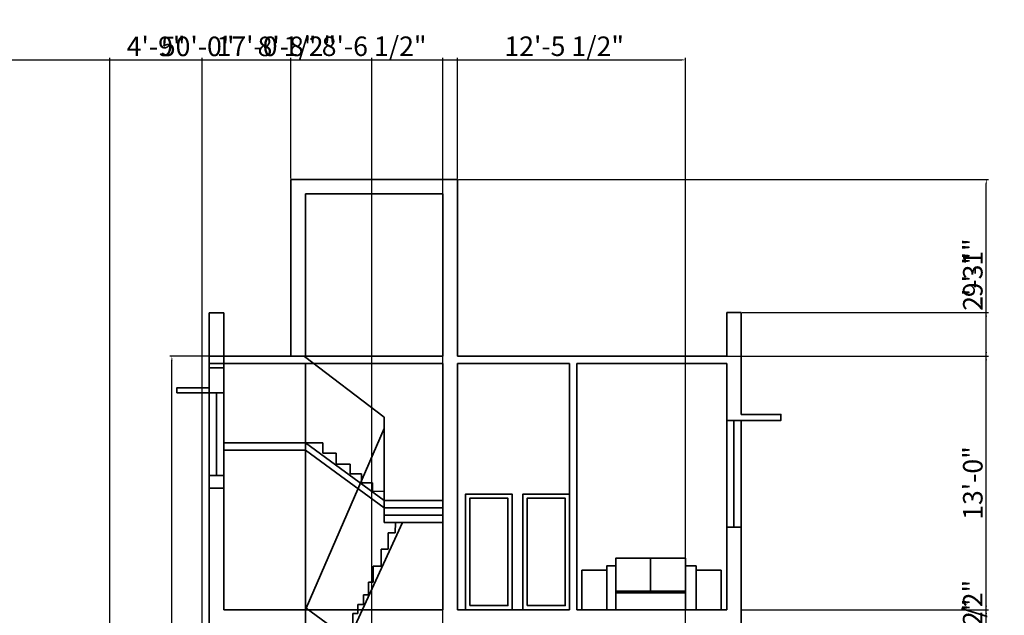
# Model space of a CAD drawing. Units: inches. Extents: x 1367 to 2309, y 1406 to 3826.
# Tile 9 of 9: x 1704 to 2309, y 3460 to 3826. Entities that reach past the tile are written whole.
import ezdxf

# ---------------------------------------------------------------- set-up
doc = ezdxf.new("R2010")
doc.units = ezdxf.units.IN
doc.layers.add('A-ANNO-DIMS', color=2, linetype='Continuous', lineweight=18)
doc.layers.add('A-SECT', color=7, linetype='Continuous', lineweight=35)
doc.styles.get("Standard").update_dxf_attribs({"font": 'arial.ttf'})
doc.dimstyles.new('ISO-25', dxfattribs={"dimtxt": 12, "dimasz": 2.5, "dimexe": 1.25, "dimexo": 0.625, "dimtad": 1, "dimdec": 0, "dimlunit": 4, "dimtxsty": 'Standard', "dimcen": 2.5, "dimadec": 0, "dimazin": 0, "dimtfac": 1, "dimtdec": 0, "dimtmove": 0, "dimatfit": 3, "dimfxl": 1, "dimarcsym": 0})

# ---------------------------------------------------------------- blocks, each defined once
blk = doc.blocks.new('*D42')
at = {"layer": 'A-ANNO-DIMS', "color": 0, "lineweight": -2, "transparency": 16777216}
for p, q in [((1819.79, 3619.06), (1796.28, 3619.06)), ((1797.53, 3153.56), (1797.53, 3616.56)), ((1819.79, 3151.06), (1796.28, 3151.06))]:
    blk.add_line(p, q, dxfattribs=at)
at = {"layer": 'A-ANNO-DIMS', "color": 0, "lineweight": 100, "transparency": 16777216}
for points in [[(1797.12, 3616.56), (1797.95, 3616.56), (1797.53, 3619.06)], [(1797.12, 3153.56), (1797.95, 3153.56), (1797.53, 3151.06)]]:
    blk.add_solid(points, dxfattribs=at)
at = {"layer": 'Defpoints', "color": 0, "lineweight": 100, "transparency": 16777216}
for p in [(1797.53, 3619.06), (1820.42, 3619.06), (1820.42, 3151.06)]:
    blk.add_point(p, dxfattribs=at)
at = {"layer": 'A-ANNO-DIMS', "color": 0, "transparency": 16777216, "insert": (1790.78, 3385.06), "char_height": 12, "attachment_point": 5, "rotation": 90}
blk.add_mtext("39'", dxfattribs=at)
blk = doc.blocks.new('*D87')
at = {"layer": 'A-ANNO-DIMS', "color": 0, "lineweight": -2, "transparency": 16777216}
for p, q in [((1513.37, 2814.79), (1513.37, 3802.6)), ((2113.4, 2814.79), (2113.4, 3802.6)), ((1515.87, 3801.35), (2110.9, 3801.35))]:
    blk.add_line(p, q, dxfattribs=at)
at = {"layer": 'A-ANNO-DIMS', "color": 0, "lineweight": 100, "transparency": 16777216}
for points in [[(1515.87, 3801.77), (1515.87, 3800.93), (1513.37, 3801.35)], [(2110.9, 3801.77), (2110.9, 3800.93), (2113.4, 3801.35)]]:
    blk.add_solid(points, dxfattribs=at)
at = {"layer": 'Defpoints', "color": 0, "lineweight": 100, "transparency": 16777216}
for p in [(2113.4, 3801.35), (1513.37, 2814.17), (2113.4, 2814.17)]:
    blk.add_point(p, dxfattribs=at)
at = {"layer": 'A-ANNO-DIMS', "color": 0, "transparency": 16777216, "insert": (1813.39, 3808.1), "char_height": 12, "attachment_point": 5}
blk.add_mtext('50\'-0"', dxfattribs=at)
blk = doc.blocks.new('*D103')
at = {"layer": 'A-ANNO-DIMS', "color": 0, "lineweight": -2, "transparency": 16777216}
for p, q in [((1504.37, 3284.24), (1504.37, 3802.6)), ((1759.42, 3284.24), (1759.42, 3802.6)), ((1506.87, 3801.35), (1756.92, 3801.35))]:
    blk.add_line(p, q, dxfattribs=at)
at = {"layer": 'A-ANNO-DIMS', "color": 0, "lineweight": 100, "transparency": 16777216}
for points in [[(1506.87, 3801.77), (1506.87, 3800.93), (1504.37, 3801.35)], [(1756.92, 3801.77), (1756.92, 3800.93), (1759.42, 3801.35)]]:
    blk.add_solid(points, dxfattribs=at)
at = {"layer": 'Defpoints', "color": 0, "lineweight": 100, "transparency": 16777216}
for p in [(1759.42, 3801.35), (1504.37, 3283.62), (1759.42, 3283.62)]:
    blk.add_point(p, dxfattribs=at)
at = {"layer": 'A-ANNO-DIMS', "color": 0, "transparency": 16777216, "insert": (1631.89, 3808.1), "char_height": 12, "attachment_point": 5}
blk.add_mtext('21\'-3"', dxfattribs=at)
blk = doc.blocks.new('*D106')
at = {"layer": 'A-ANNO-DIMS', "color": 0, "lineweight": -2, "transparency": 16777216}
for p, q in [((1759.42, 3063.31), (1759.42, 3802.6)), ((1964.13, 3080.24), (1964.13, 3802.6)), ((1761.92, 3801.35), (1961.63, 3801.35))]:
    blk.add_line(p, q, dxfattribs=at)
at = {"layer": 'A-ANNO-DIMS', "color": 0, "lineweight": 100, "transparency": 16777216}
for points in [[(1761.92, 3801.77), (1761.92, 3800.93), (1759.42, 3801.35)], [(1961.63, 3801.77), (1961.63, 3800.93), (1964.13, 3801.35)]]:
    blk.add_solid(points, dxfattribs=at)
at = {"layer": 'Defpoints', "color": 0, "lineweight": 100, "transparency": 16777216}
for p in [(1964.13, 3801.35), (1964.13, 3079.62), (1759.42, 3062.68)]:
    blk.add_point(p, dxfattribs=at)
at = {"layer": 'A-ANNO-DIMS', "color": 0, "transparency": 16777216, "insert": (1861.77, 3808.18), "char_height": 12, "attachment_point": 5}
blk.add_mtext('17\'-0 1/2"', dxfattribs=at)
blk = doc.blocks.new('*D107')
at = {"layer": 'A-ANNO-DIMS', "color": 0, "lineweight": -2, "transparency": 16777216}
for p, q in [((1964.13, 3080.24), (1964.13, 3802.6)), ((2113.4, 3080.24), (2113.4, 3802.6)), ((1966.63, 3801.35), (2110.9, 3801.35))]:
    blk.add_line(p, q, dxfattribs=at)
at = {"layer": 'A-ANNO-DIMS', "color": 0, "lineweight": 100, "transparency": 16777216}
for points in [[(1966.63, 3801.77), (1966.63, 3800.93), (1964.13, 3801.35)], [(2110.9, 3801.77), (2110.9, 3800.93), (2113.4, 3801.35)]]:
    blk.add_solid(points, dxfattribs=at)
at = {"layer": 'Defpoints', "color": 0, "lineweight": 100, "transparency": 16777216}
for p in [(2113.4, 3801.35), (1964.13, 3079.62), (2113.4, 3079.62)]:
    blk.add_point(p, dxfattribs=at)
at = {"layer": 'A-ANNO-DIMS', "color": 0, "transparency": 16777216, "insert": (2038.76, 3808.18), "char_height": 12, "attachment_point": 5}
blk.add_mtext('12\'-5 1/2"', dxfattribs=at)
blk = doc.blocks.new('*D110')
at = {"layer": 'A-ANNO-DIMS', "color": 0, "lineweight": -2, "transparency": 16777216}
for p, q in [((1816.25, 3045.71), (1816.25, 3802.6)), ((1920.42, 3047.12), (1920.42, 3802.6)), ((1818.75, 3801.35), (1917.92, 3801.35))]:
    blk.add_line(p, q, dxfattribs=at)
at = {"layer": 'A-ANNO-DIMS', "color": 0, "lineweight": 100, "transparency": 16777216}
for points in [[(1818.75, 3801.77), (1818.75, 3800.93), (1816.25, 3801.35)], [(1917.92, 3801.77), (1917.92, 3800.93), (1920.42, 3801.35)]]:
    blk.add_solid(points, dxfattribs=at)
at = {"layer": 'Defpoints', "color": 0, "lineweight": 100, "transparency": 16777216}
for p in [(1920.42, 3801.35), (1816.25, 3045.09), (1920.42, 3046.5)]:
    blk.add_point(p, dxfattribs=at)
at = {"layer": 'A-ANNO-DIMS', "color": 0, "transparency": 16777216, "insert": (1868.33, 3808.1), "char_height": 12, "attachment_point": 5}
blk.add_mtext('8\'-8"', dxfattribs=at)
blk = doc.blocks.new('*D111')
at = {"layer": 'A-ANNO-DIMS', "color": 0, "lineweight": -2, "transparency": 16777216}
for p, q in [((1759.42, 3063.31), (1759.42, 3802.6)), ((1816.25, 3063.31), (1816.25, 3802.6)), ((1761.92, 3801.35), (1813.75, 3801.35))]:
    blk.add_line(p, q, dxfattribs=at)
at = {"layer": 'A-ANNO-DIMS', "color": 0, "lineweight": 100, "transparency": 16777216}
for points in [[(1761.92, 3801.77), (1761.92, 3800.93), (1759.42, 3801.35)], [(1813.75, 3801.77), (1813.75, 3800.93), (1816.25, 3801.35)]]:
    blk.add_solid(points, dxfattribs=at)
at = {"layer": 'Defpoints', "color": 0, "lineweight": 100, "transparency": 16777216}
for p in [(1816.25, 3801.35), (1759.42, 3062.68), (1816.25, 3062.68)]:
    blk.add_point(p, dxfattribs=at)
at = {"layer": 'A-ANNO-DIMS', "color": 0, "transparency": 16777216, "insert": (1787.83, 3808.1), "char_height": 12, "attachment_point": 5}
blk.add_mtext('4\'-9"', dxfattribs=at)
blk = doc.blocks.new('*D118')
at = {"layer": 'A-ANNO-DIMS', "color": 0, "lineweight": -2, "transparency": 16777216}
for p, q in [((1973.75, 3727.85), (2299.51, 3727.85)), ((2298.26, 3132.02), (2298.26, 3725.35)), ((2211.02, 3129.52), (2299.51, 3129.52))]:
    blk.add_line(p, q, dxfattribs=at)
at = {"layer": 'A-ANNO-DIMS', "color": 0, "lineweight": 100, "transparency": 16777216}
for points in [[(2297.84, 3725.35), (2298.67, 3725.35), (2298.26, 3727.85)], [(2297.84, 3132.02), (2298.67, 3132.02), (2298.26, 3129.52)]]:
    blk.add_solid(points, dxfattribs=at)
at = {"layer": 'Defpoints', "color": 0, "lineweight": 100, "transparency": 16777216}
for p in [(1973.13, 3727.85), (2298.26, 3727.85), (2210.4, 3129.52)]:
    blk.add_point(p, dxfattribs=at)
at = {"layer": 'A-ANNO-DIMS', "color": 0, "transparency": 16777216, "insert": (2291.43, 3428.69), "char_height": 12, "attachment_point": 5, "rotation": 90}
blk.add_mtext('49\'-10 1/2"', dxfattribs=at)
blk = doc.blocks.new('*D120')
at = {"layer": 'A-ANNO-DIMS', "color": 0, "lineweight": -2, "transparency": 16777216}
for p, q in [((2148.26, 3463.06), (2299.51, 3463.06)), ((2298.26, 3309.56), (2298.26, 3460.56)), ((2148.26, 3307.06), (2299.51, 3307.06))]:
    blk.add_line(p, q, dxfattribs=at)
at = {"layer": 'A-ANNO-DIMS', "color": 0, "lineweight": 100, "transparency": 16777216}
for points in [[(2297.84, 3460.56), (2298.67, 3460.56), (2298.26, 3463.06)], [(2297.84, 3309.56), (2298.67, 3309.56), (2298.26, 3307.06)]]:
    blk.add_solid(points, dxfattribs=at)
at = {"layer": 'Defpoints', "color": 0, "lineweight": 100, "transparency": 16777216}
for p in [(2147.64, 3463.06), (2298.26, 3463.06), (2147.64, 3307.06)]:
    blk.add_point(p, dxfattribs=at)
at = {"layer": 'A-ANNO-DIMS', "color": 0, "transparency": 16777216, "insert": (2291.5, 3385.06), "char_height": 12, "attachment_point": 5, "rotation": 90}
blk.add_mtext('13\'-0"', dxfattribs=at)
blk = doc.blocks.new('*D121')
at = {"layer": 'A-ANNO-DIMS', "color": 0, "lineweight": -2, "transparency": 16777216}
for p, q in [((2148.26, 3619.06), (2299.51, 3619.06)), ((2298.26, 3465.56), (2298.26, 3616.56)), ((2148.26, 3463.06), (2299.51, 3463.06))]:
    blk.add_line(p, q, dxfattribs=at)
at = {"layer": 'A-ANNO-DIMS', "color": 0, "lineweight": 100, "transparency": 16777216}
for points in [[(2297.84, 3616.56), (2298.67, 3616.56), (2298.26, 3619.06)], [(2297.84, 3465.56), (2298.67, 3465.56), (2298.26, 3463.06)]]:
    blk.add_solid(points, dxfattribs=at)
at = {"layer": 'Defpoints', "color": 0, "lineweight": 100, "transparency": 16777216}
for p in [(2147.64, 3619.06), (2298.26, 3619.06), (2147.64, 3463.06)]:
    blk.add_point(p, dxfattribs=at)
at = {"layer": 'A-ANNO-DIMS', "color": 0, "transparency": 16777216, "insert": (2291.5, 3541.06), "char_height": 12, "attachment_point": 5, "rotation": 90}
blk.add_mtext('13\'-0"', dxfattribs=at)
blk = doc.blocks.new('*D122')
at = {"layer": 'A-ANNO-DIMS', "color": 0, "lineweight": -2, "transparency": 16777216}
for p, q in [((2298.26, 3645.91), (2298.26, 3681.76)), ((2148.26, 3645.91), (2299.51, 3645.91)), ((2298.26, 3621.56), (2298.26, 3643.41)), ((2148.26, 3619.06), (2299.51, 3619.06))]:
    blk.add_line(p, q, dxfattribs=at)
at = {"layer": 'A-ANNO-DIMS', "color": 0, "lineweight": 100, "transparency": 16777216}
for points in [[(2297.84, 3643.41), (2298.67, 3643.41), (2298.26, 3645.91)], [(2297.84, 3621.56), (2298.67, 3621.56), (2298.26, 3619.06)]]:
    blk.add_solid(points, dxfattribs=at)
at = {"layer": 'Defpoints', "color": 0, "lineweight": 100, "transparency": 16777216}
for p in [(2147.64, 3645.91), (2298.26, 3645.91), (2147.64, 3619.06)]:
    blk.add_point(p, dxfattribs=at)
at = {"layer": 'A-ANNO-DIMS', "color": 0, "transparency": 16777216, "insert": (2291.5, 3665.09), "char_height": 12, "attachment_point": 5, "rotation": 90}
blk.add_mtext('2\'-3"', dxfattribs=at)
blk = doc.blocks.new('*D123')
at = {"layer": 'A-ANNO-DIMS', "color": 0, "lineweight": -2, "transparency": 16777216}
for p, q in [((1973.75, 3727.85), (2299.51, 3727.85)), ((2298.26, 3621.56), (2298.26, 3725.35)), ((1973.75, 3619.06), (2299.51, 3619.06))]:
    blk.add_line(p, q, dxfattribs=at)
at = {"layer": 'A-ANNO-DIMS', "color": 0, "lineweight": 100, "transparency": 16777216}
for points in [[(2297.84, 3725.35), (2298.67, 3725.35), (2298.26, 3727.85)], [(2297.84, 3621.56), (2298.67, 3621.56), (2298.26, 3619.06)]]:
    blk.add_solid(points, dxfattribs=at)
at = {"layer": 'Defpoints', "color": 0, "lineweight": 100, "transparency": 16777216}
for p in [(1973.13, 3727.85), (2298.26, 3727.85), (1973.13, 3619.06)]:
    blk.add_point(p, dxfattribs=at)
at = {"layer": 'A-ANNO-DIMS', "color": 0, "transparency": 16777216, "insert": (2291.51, 3673.46), "char_height": 12, "attachment_point": 5, "rotation": 90}
blk.add_mtext('9\'-1"', dxfattribs=at)
blk = doc.blocks.new('*D125')
at = {"layer": 'A-ANNO-DIMS', "color": 0, "lineweight": -2, "transparency": 16777216}
for p, q in [((1870.66, 3728.47), (1870.66, 3802.6)), ((1973.13, 3728.47), (1973.13, 3802.6)), ((1873.16, 3801.35), (1970.63, 3801.35))]:
    blk.add_line(p, q, dxfattribs=at)
at = {"layer": 'A-ANNO-DIMS', "color": 0, "lineweight": 100, "transparency": 16777216}
for points in [[(1873.16, 3801.77), (1873.16, 3800.93), (1870.66, 3801.35)], [(1970.63, 3801.77), (1970.63, 3800.93), (1973.13, 3801.35)]]:
    blk.add_solid(points, dxfattribs=at)
at = {"layer": 'Defpoints', "color": 0, "lineweight": 100, "transparency": 16777216}
for p in [(1973.13, 3801.35), (1870.66, 3727.85), (1973.13, 3727.85)]:
    blk.add_point(p, dxfattribs=at)
at = {"layer": 'A-ANNO-DIMS', "color": 0, "transparency": 16777216, "insert": (1921.89, 3808.18), "char_height": 12, "attachment_point": 5}
blk.add_mtext('8\'-6 1/2"', dxfattribs=at)
blk = doc.blocks.new('*D134')
at = {"layer": 'A-ANNO-DIMS', "color": 0, "lineweight": -2, "transparency": 16777216}
for p, q in [((2298.26, 3416.79), (2298.26, 3479.27)), ((1649.56, 3416.79), (2299.51, 3416.79)), ((2298.26, 3399.83), (2298.26, 3414.29)), ((1649.56, 3397.33), (2299.51, 3397.33))]:
    blk.add_line(p, q, dxfattribs=at)
at = {"layer": 'A-ANNO-DIMS', "color": 0, "lineweight": 100, "transparency": 16777216}
for points in [[(2297.84, 3414.29), (2298.67, 3414.29), (2298.26, 3416.79)], [(2297.84, 3399.83), (2298.67, 3399.83), (2298.26, 3397.33)]]:
    blk.add_solid(points, dxfattribs=at)
at = {"layer": 'Defpoints', "color": 0, "lineweight": 100, "transparency": 16777216}
for p in [(1648.94, 3416.79), (2298.26, 3416.79), (1648.94, 3397.33)]:
    blk.add_point(p, dxfattribs=at)
at = {"layer": 'A-ANNO-DIMS', "color": 0, "transparency": 16777216, "insert": (2291.43, 3449.28), "char_height": 12, "attachment_point": 5, "rotation": 90}
blk.add_mtext('1\'-7 1/2"', dxfattribs=at)

msp = doc.modelspace()

# ---------------------------------------------------------------- linework, layer by layer
at = {"layer": 'A-SECT'}
for p, q in [((1870.66, 3619.06), (1870.66, 3727.85)), ((1870.66, 3727.85), (1973.13, 3727.85)), ((1973.13, 3619.06), (1973.13, 3727.85)), ((1879.66, 3718.85), (1964.13, 3718.85)), ((1879.66, 3618.43), (1879.66, 3718.85)), ((1964.13, 3619.06), (1964.13, 3718.85)), ((1829.42, 3645.66), (1820.42, 3645.66)), ((1820.42, 3645.66), (1820.42, 3604.46)), ((1829.42, 3463.06), (1829.42, 3645.66)), ((2138.64, 3645.91), (2147.64, 3645.91)), ((2138.64, 3619.06), (2138.64, 3645.91)), ((2147.64, 3645.91), (2147.64, 3609.4)), ((1820.42, 3463.06), (1820.42, 3619.06)), ((1820.42, 3619.06), (1964.13, 3619.06)), ((1820.42, 3614.56), (1964.13, 3614.56)), ((1879.13, 3618.83), (1928.13, 3581.56)), ((1879.66, 3151.06), (1879.66, 3614.56)), ((1964.13, 3463.06), (1964.13, 3614.56)), ((1973.13, 3619.06), (2138.64, 3619.06)), ((1973.13, 3614.56), (2041.96, 3614.56)), ((1973.13, 3463.06), (1973.13, 3614.56)), ((2041.96, 3463.06), (2041.96, 3614.56)), ((2046.46, 3614.56), (2138.64, 3614.56)), ((2046.46, 3463.06), (2046.46, 3614.56)), ((2138.64, 3463.06), (2138.64, 3614.56)), ((2147.64, 3619.06), (2147.64, 3583.3)), ((1824.92, 3596.6), (1824.92, 3545.64)), ((1928.13, 3530.25), (1928.13, 3581.56)), ((2143.14, 3579.56), (2143.14, 3514)), ((2147.64, 3579.56), (2147.64, 3454.43)), ((1880.03, 3464.13), (1928.13, 3574.55)), ((1829.42, 3565.74), (1879.66, 3565.74)), ((1879.66, 3565.74), (1928.13, 3530.25)), ((1879.66, 3565.74), (1890.3, 3565.74)), ((1890.3, 3565.74), (1890.3, 3559.32)), ((1829.42, 3561.24), (1879.66, 3561.24)), ((1879.66, 3561.24), (1928.13, 3525.75)), ((1890.3, 3559.32), (1898.59, 3559.32)), ((1898.59, 3559.32), (1898.59, 3552.63)), ((1898.59, 3552.63), (1907.23, 3552.63)), ((1907.23, 3552.63), (1907.23, 3546.73)), ((1907.23, 3546.73), (1914.17, 3546.73)), ((1914.17, 3546.73), (1914.17, 3541.26)), ((1914.17, 3541.26), (1920.94, 3541.26)), ((1920.94, 3541.26), (1920.94, 3536.05)), ((1920.94, 3536.05), (1928.13, 3535.83)), ((1964.13, 3530.25), (1928.13, 3530.25)), ((1928.13, 3516.75), (1928.13, 3530.25)), ((1964.13, 3525.75), (1928.13, 3525.75)), ((1964.13, 3521.25), (1928.13, 3521.25)), ((1881.33, 3390.43), (1939.32, 3516.75)), ((1964.13, 3516.75), (1928.13, 3516.75)), ((1934.86, 3510.47), (1935.02, 3516.75)), ((1930.51, 3500.3), (1930.51, 3510.47)), ((1930.51, 3510.47), (1934.86, 3510.47)), ((1926.3, 3489.93), (1926.3, 3500.3)), ((1926.3, 3500.3), (1930.51, 3500.3)), ((2091.9, 3494.86), (2091.9, 3474.61)), ((1921.39, 3479.98), (1921.39, 3489.93)), ((1921.39, 3489.93), (1926.3, 3489.93)), ((1918.41, 3472.3), (1918.41, 3479.98)), ((1918.41, 3479.98), (1921.39, 3479.98)), ((2070.5, 3474.61), (2113.29, 3474.61)), ((1915.43, 3466.42), (1915.43, 3472.3)), ((1915.43, 3472.3), (1918.41, 3472.3)), ((2070.5, 3473.59), (2113.29, 3473.59)), ((1820.42, 3307.06), (1820.42, 3463.06)), ((1829.42, 3463.06), (1964.13, 3463.06)), ((1880.03, 3464.13), (1928.13, 3428.92)), ((1911.93, 3460.79), (1911.93, 3466.42)), ((1911.93, 3466.42), (1915.43, 3466.42)), ((1973.13, 3463.06), (2041.96, 3463.06)), ((2046.46, 3463.06), (2138.64, 3463.06)), ((2147.64, 3463.06), (2147.64, 3307.06)), ((1908.8, 3451.94), (1908.8, 3460.79)), ((1908.8, 3460.79), (1911.93, 3460.79))]:
    msp.add_line(p, q, dxfattribs=at)
for points in [[(1820.42, 3537.94), (1829.42, 3537.94), (1829.42, 3611.88), (1820.42, 3611.88)], [(1820.42, 3596.6), (1800.63, 3596.6), (1800.63, 3599.61), (1820.42, 3599.61)], [(1820.42, 3596.6), (1829.42, 3596.6), (1829.42, 3545.64), (1820.42, 3545.64)], [(2138.64, 3579.56), (2147.64, 3579.56), (2147.64, 3514), (2138.64, 3514)], [(1978.13, 3463.06), (2006.73, 3463.06), (2006.73, 3534.26), (1978.13, 3534.26)], [(1980.73, 3465.66), (2004.13, 3465.66), (2004.13, 3531.66), (1980.73, 3531.66)], [(2013.36, 3463.06), (2041.96, 3463.06), (2041.96, 3534.26), (2013.36, 3534.26)], [(2015.96, 3465.66), (2039.36, 3465.66), (2039.36, 3531.66), (2015.96, 3531.66)], [(2070.5, 3463.06), (2113.29, 3463.06), (2113.29, 3494.86), (2070.5, 3494.86)], [(2049.59, 3463.06), (2064.95, 3463.06), (2064.95, 3487.35), (2049.59, 3487.35)], [(2070.5, 3490.08), (2064.95, 3490.08), (2064.95, 3463.06), (2070.5, 3463.06)], [(2119.87, 3490.08), (2113.29, 3490.13), (2113.29, 3463.11), (2119.87, 3463.06)], [(2119.87, 3463.06), (2135.22, 3463.06), (2135.22, 3487.35), (2119.87, 3487.35)]]:
    msp.add_lwpolyline(points, close=True, dxfattribs=at)
msp.add_lwpolyline([(2147.64, 3579.56), (2172.02, 3579.56), (2172.02, 3583.3), (2147.64, 3583.3)], dxfattribs=at)

# ---------------------------------------------------------------- dimensions: what is measured, and where the dimension line sits
at = {"layer": 'A-ANNO-DIMS'}
for base, p1, p2, picture, middle in [((1964.13, 3801.35), (1759.42, 3062.68), (1964.13, 3079.62), '*D106', (1861.77, 3808.18)), ((1973.13, 3801.35), (1870.66, 3727.85), (1973.13, 3727.85), '*D125', (1921.89, 3808.18)), ((2113.4, 3801.35), (1964.13, 3079.62), (2113.4, 3079.62), '*D107', (2038.76, 3808.18)), ((1759.4169, 3801.349), (1504.3701, 3283.618), (1759.4169, 3283.618), '*D103', (1631.8935, 3808.105)), ((2113.4, 3801.35), (1513.37, 2814.17), (2113.4, 2814.17), '*D87', (1813.39, 3808.1)), ((1816.25, 3801.35), (1759.42, 3062.68), (1816.25, 3062.68), '*D111', (1787.83, 3808.1)), ((1920.42, 3801.35), (1816.25, 3045.09), (1920.42, 3046.5), '*D110', (1868.33, 3808.1))]:
    dim = msp.add_linear_dim(base=base, p1=p1, p2=p2, dimstyle='ISO-25', override={"dimdec": 1, "dimlfac": 1, "dimrnd": 0, "dimzin": 1, "dimdsep": 46, "dimlunit": 4, "dimfrac": 2}, dxfattribs=at)
    dim.commit()
    dim.dimension.update_dxf_attribs({"geometry": picture, "text_midpoint": middle})
for base, p1, p2, override, picture, middle in [((2298.26, 3727.85), (2210.4, 3129.52), (1973.13, 3727.85), {"dimdec": 1, "dimlfac": 1, "dimrnd": 0, "dimzin": 1, "dimdsep": 46, "dimlunit": 4, "dimfrac": 2}, '*D118', (2291.43, 3428.69)), ((2298.26, 3727.85), (1973.13, 3619.06), (1973.13, 3727.85), {"dimdec": 1, "dimlfac": 1, "dimrnd": 0, "dimzin": 1, "dimdsep": 46, "dimlunit": 4, "dimfrac": 2}, '*D123', (2291.51, 3673.46)), ((2298.2577, 3645.9083), (2147.6368, 3619.0644), (2147.6368, 3645.9083), {"dimdec": 1, "dimlfac": 1, "dimrnd": 0, "dimzin": 1, "dimdsep": 46, "dimlunit": 4, "dimfrac": 2}, '*D122', (2291.5018, 3665.0851)), ((1797.53, 3619.06), (1820.42, 3151.06), (1820.42, 3619.06), {"dimclrd": 0, "dimclre": 0, "dimclrt": 0}, '*D42', (1790.78, 3385.06)), ((2298.26, 3619.06), (2147.64, 3463.06), (2147.64, 3619.06), {"dimdec": 1, "dimlfac": 1, "dimrnd": 0, "dimzin": 1, "dimdsep": 46, "dimlunit": 4, "dimfrac": 2}, '*D121', (2291.5, 3541.06)), ((2298.26, 3416.79), (1648.94, 3397.33), (1648.94, 3416.79), {"dimdec": 1, "dimlfac": 1, "dimrnd": 0, "dimzin": 1, "dimdsep": 46, "dimlunit": 4, "dimfrac": 2}, '*D134', (2291.43, 3449.28)), ((2298.26, 3463.06), (2147.64, 3307.06), (2147.64, 3463.06), {"dimdec": 1, "dimlfac": 1, "dimrnd": 0, "dimzin": 1, "dimdsep": 46, "dimlunit": 4, "dimfrac": 2}, '*D120', (2291.5, 3385.06))]:
    dim = msp.add_linear_dim(base=base, p1=p1, p2=p2, angle=90, dimstyle='ISO-25', override=override, dxfattribs=at)
    dim.commit()
    dim.dimension.update_dxf_attribs({"geometry": picture, "text_midpoint": middle})

doc.saveas('drawing.dxf')
